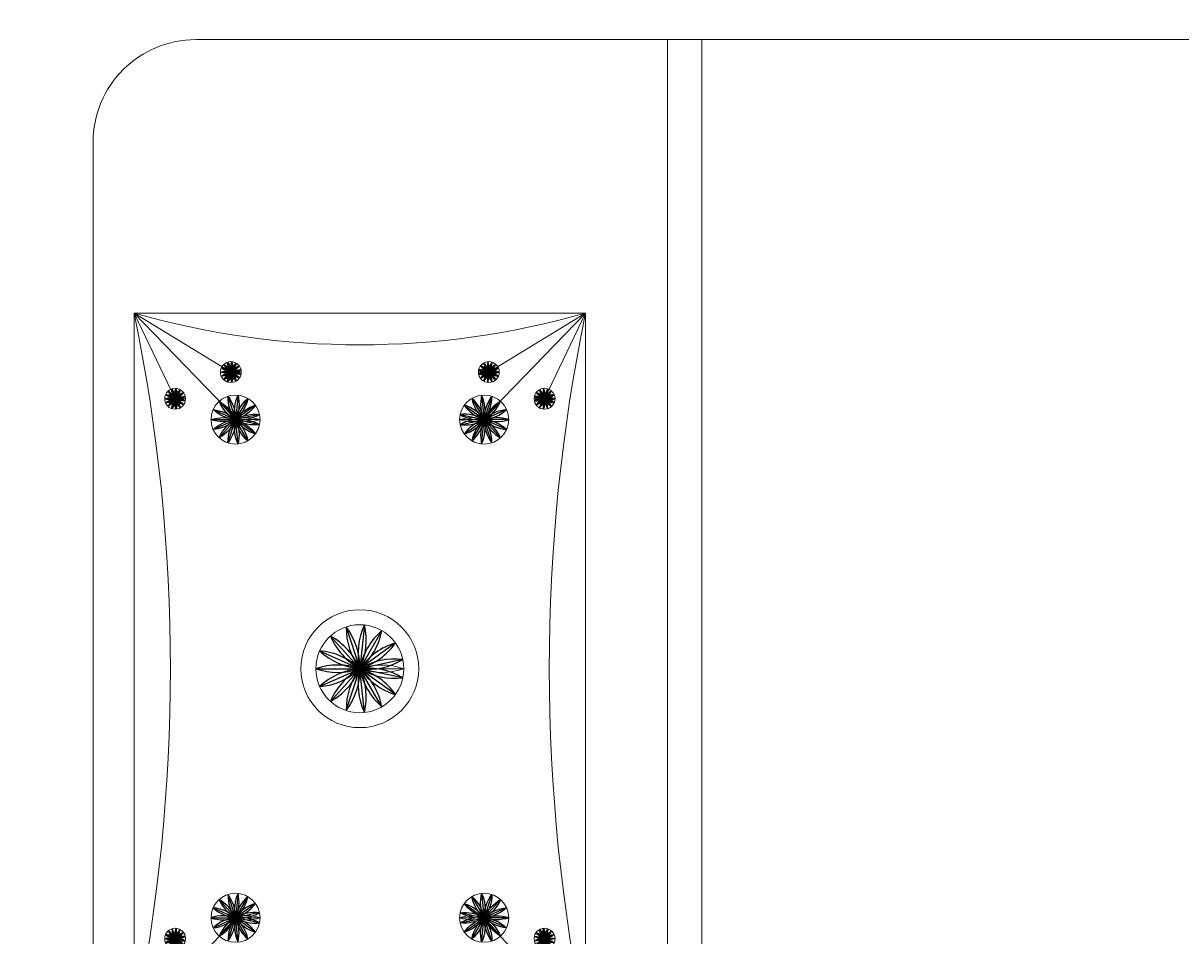
# Model space of a CAD drawing. Units: inches. Extents: x -61 to 1599, y -1316 to 257.
# Tile 149 of 204: x 406 to 440, y 101 to 127. Entities that reach past the tile are written whole.
import ezdxf

# ---------------------------------------------------------------- set-up
doc = ezdxf.new("R2010")
doc.units = ezdxf.units.IN
doc.header["$MEASUREMENT"] = 0
doc.layers.add('A-ANNO-DIMS', color=2, linetype='Continuous', lineweight=18)
doc.layers.add('FURNITURE', color=83, linetype='Continuous', lineweight=18)
doc.layers.add('LT', color=8, linetype='Continuous')
doc.styles.get("Standard").update_dxf_attribs({"font": 'arial.ttf'})
doc.dimstyles.get("Standard").update_dxf_attribs({"dimtxt": 0.18, "dimasz": 0.18, "dimexe": 0.18, "dimexo": 0.0625, "dimgap": 0.09, "dimtad": 0, "dimtih": 1, "dimtoh": 1, "dimdec": 0, "dimzin": 0, "dimdsep": 46, "dimlunit": 3, "dimtxsty": 'Standard', "dimcen": 0.09, "dimadec": 0, "dimazin": 0, "dimtfac": 1, "dimtdec": 0, "dimtofl": 0, "dimtmove": 0, "dimatfit": 3, "dimfxl": 1, "dimtolj": 1, "dimtzin": 0, "dimarcsym": 0})

# ---------------------------------------------------------------- blocks, each defined once
blk = doc.blocks.new('*U71')
at = {"layer": 'LT'}
blk.add_line((0, 0.152), (0, -0.152), dxfattribs=at)
for centre, start, end in [((0.443, 0), 160.9983, 199.0017), ((-0.443, 0), 340.9983, 19.0017)]:
    blk.add_arc(centre, 0.468, start, end, dxfattribs=at)
blk = doc.blocks.new('*U58')
at = {"layer": 'LT', "transparency": 16777216}
for p, rotation in [((-57.958, -16.311), 72), ((-57.926, -16.256), 48.00000000000001), ((-57.875, -16.219), 24), ((-57.751, -16.219), 336), ((-57.699, -16.256), 312), ((-57.668, -16.311), 288), ((-57.964, -16.374), 96), ((-57.945, -16.435), 120), ((-57.902, -16.482), 144), ((-57.844, -16.508), 168.0000000000001), ((-57.781, -16.508), 192), ((-57.723, -16.482), 216), ((-57.68, -16.435), 240), ((-57.661, -16.374), 264)]:
    blk.add_blockref('*U71', p, dxfattribs=dict(at, rotation=rotation))
blk.add_blockref('*U71', (-57.813, -16.206), dxfattribs=at)
blk = doc.blocks.new('*U61')
at = {"layer": 'LT'}
blk.add_line((0, 0.152), (0, -0.152), dxfattribs=at)
for centre, start, end in [((0.443, 0), 160.9983, 199.0017), ((-0.443, 0), 340.9983, 19.0017)]:
    blk.add_arc(centre, 0.468, start, end, dxfattribs=at)
blk = doc.blocks.new('*U62')
at = {"layer": 'LT', "transparency": 16777216}
for p, rotation in [((-57.958, -16.311), 72), ((-57.926, -16.256), 48.00000000000001), ((-57.875, -16.219), 24), ((-57.751, -16.219), 336), ((-57.699, -16.256), 312), ((-57.668, -16.311), 288), ((-57.964, -16.374), 96), ((-57.945, -16.435), 120), ((-57.902, -16.482), 144), ((-57.844, -16.508), 168.0000000000001), ((-57.781, -16.508), 192), ((-57.723, -16.482), 216), ((-57.68, -16.435), 240), ((-57.661, -16.374), 264)]:
    blk.add_blockref('*U61', p, dxfattribs=dict(at, rotation=rotation))
blk.add_blockref('*U61', (-57.813, -16.206), dxfattribs=at)
blk = doc.blocks.new('*U80')
at = {"layer": 'LT'}
blk.add_line((0, 0.359), (0, -0.359), dxfattribs=at)
for centre, start, end in [((1.041, 0), 160.9983, 199.0017), ((-1.041, 0), 340.9983, 19.0017)]:
    blk.add_arc(centre, 1.101, start, end, dxfattribs=at)
blk = doc.blocks.new('*U96')
at = {"layer": 'LT', "transparency": 16777216}
for p, rotation in [((-136.107, -38.143), 23.99999999999999), ((-135.815, -38.143), 336.0000000000001), ((-136.302, -38.36), 72), ((-136.227, -38.231), 48.00000000000001), ((-135.694, -38.231), 312), ((-135.62, -38.36), 288.0000000000001), ((-136.318, -38.508), 96), ((-136.271, -38.65), 120), ((-136.172, -38.761), 144), ((-136.035, -38.822), 168.0000000000001), ((-135.886, -38.822), 191.9999999999999), ((-135.75, -38.761), 216), ((-135.65, -38.65), 240), ((-135.604, -38.508), 264)]:
    blk.add_blockref('*U80', p, dxfattribs=dict(at, rotation=rotation))
blk.add_blockref('*U80', (-135.961, -38.112), dxfattribs=at)
blk = doc.blocks.new('*U69')
at = {"layer": 'LT'}
blk.add_line((0, 0.359), (0, -0.359), dxfattribs=at)
for centre, start, end in [((1.041, 0), 160.9983, 199.0017), ((-1.041, 0), 340.9983, 19.0017)]:
    blk.add_arc(centre, 1.101, start, end, dxfattribs=at)
blk = doc.blocks.new('*U70')
at = {"layer": 'LT', "transparency": 16777216}
for p, rotation in [((-136.107, -38.143), 23.99999999999999), ((-135.815, -38.143), 336.0000000000001), ((-136.302, -38.36), 72), ((-136.227, -38.231), 48.00000000000001), ((-135.694, -38.231), 312), ((-135.62, -38.36), 288.0000000000001), ((-136.318, -38.508), 96), ((-136.271, -38.65), 120), ((-136.172, -38.761), 144), ((-136.035, -38.822), 168.0000000000001), ((-135.886, -38.822), 191.9999999999999), ((-135.75, -38.761), 216), ((-135.65, -38.65), 240), ((-135.604, -38.508), 264)]:
    blk.add_blockref('*U69', p, dxfattribs=dict(at, rotation=rotation))
blk.add_blockref('*U69', (-135.961, -38.112), dxfattribs=at)
blk = doc.blocks.new('*U67')
at = {"layer": 'LT'}
blk.add_line((0, 0.152), (0, -0.152), dxfattribs=at)
for centre, start, end in [((0.443, 0), 160.9983, 199.0017), ((-0.443, 0), 340.9983, 19.0017)]:
    blk.add_arc(centre, 0.468, start, end, dxfattribs=at)
blk = doc.blocks.new('*U68')
at = {"layer": 'LT', "transparency": 16777216}
for p, rotation in [((-57.958, -16.311), 72), ((-57.926, -16.256), 48.00000000000001), ((-57.875, -16.219), 24), ((-57.751, -16.219), 336), ((-57.699, -16.256), 312), ((-57.668, -16.311), 288), ((-57.964, -16.374), 96), ((-57.945, -16.435), 120), ((-57.902, -16.482), 144), ((-57.844, -16.508), 168.0000000000001), ((-57.781, -16.508), 192), ((-57.723, -16.482), 216), ((-57.68, -16.435), 240), ((-57.661, -16.374), 264)]:
    blk.add_blockref('*U67', p, dxfattribs=dict(at, rotation=rotation))
blk.add_blockref('*U67', (-57.813, -16.206), dxfattribs=at)
blk = doc.blocks.new('*U63')
at = {"layer": 'LT'}
blk.add_line((0, 0.643), (0, -0.643), dxfattribs=at)
for centre, start, end in [((1.867, 0), 160.9983, 199.0017), ((-1.867, 0), 340.9983, 19.0017)]:
    blk.add_arc(centre, 1.975, start, end, dxfattribs=at)
blk = doc.blocks.new('*U64')
at = {"layer": 'LT', "transparency": 16777216}
blk.add_blockref('*U63', (-243.723, -68.32), dxfattribs=at)
for p, rotation in [((-244.201, -68.532), 48.00000000000001), ((-243.984, -68.375), 23.99999999999999), ((-243.461, -68.375), 336.0000000000001), ((-243.245, -68.532), 312), ((-244.334, -68.764), 72), ((-243.111, -68.764), 288), ((-244.362, -69.03), 96), ((-244.28, -69.284), 120), ((-244.101, -69.483), 144), ((-243.856, -69.591), 168), ((-243.589, -69.591), 192), ((-243.345, -69.483), 216), ((-243.166, -69.284), 240), ((-243.083, -69.03), 264)]:
    blk.add_blockref('*U63', p, dxfattribs=dict(at, rotation=rotation))
blk = doc.blocks.new('*U65')
at = {"layer": 'LT'}
blk.add_line((0, 0.359), (0, -0.359), dxfattribs=at)
for centre, start, end in [((1.041, 0), 160.9983, 199.0017), ((-1.041, 0), 340.9983, 19.0017)]:
    blk.add_arc(centre, 1.101, start, end, dxfattribs=at)
blk = doc.blocks.new('*U66')
at = {"layer": 'LT', "transparency": 16777216}
for p, rotation in [((-136.107, -38.143), 23.99999999999999), ((-135.815, -38.143), 336.0000000000001), ((-136.302, -38.36), 72), ((-136.227, -38.231), 48.00000000000001), ((-135.694, -38.231), 312), ((-135.62, -38.36), 288.0000000000001), ((-136.318, -38.508), 96), ((-136.271, -38.65), 120), ((-136.172, -38.761), 144), ((-136.035, -38.822), 168.0000000000001), ((-135.886, -38.822), 191.9999999999999), ((-135.75, -38.761), 216), ((-135.65, -38.65), 240), ((-135.604, -38.508), 264)]:
    blk.add_blockref('*U65', p, dxfattribs=dict(at, rotation=rotation))
blk.add_blockref('*U65', (-135.961, -38.112), dxfattribs=at)
blk = doc.blocks.new('*U85')
at = {"layer": 'LT'}
blk.add_line((0, 0.359), (0, -0.359), dxfattribs=at)
for centre, start, end in [((1.041, 0), 160.9983, 199.0017), ((-1.041, 0), 340.9983, 19.0017)]:
    blk.add_arc(centre, 1.101, start, end, dxfattribs=at)
blk = doc.blocks.new('*U86')
at = {"layer": 'LT', "transparency": 16777216}
for p, rotation in [((-136.107, -38.143), 23.99999999999999), ((-135.815, -38.143), 336.0000000000001), ((-136.302, -38.36), 72), ((-136.227, -38.231), 48.00000000000001), ((-135.694, -38.231), 312), ((-135.62, -38.36), 288.0000000000001), ((-136.318, -38.508), 96), ((-136.271, -38.65), 120), ((-136.172, -38.761), 144), ((-136.035, -38.822), 168.0000000000001), ((-135.886, -38.822), 191.9999999999999), ((-135.75, -38.761), 216), ((-135.65, -38.65), 240), ((-135.604, -38.508), 264)]:
    blk.add_blockref('*U85', p, dxfattribs=dict(at, rotation=rotation))
blk.add_blockref('*U85', (-135.961, -38.112), dxfattribs=at)
blk = doc.blocks.new('*U97')
at = {"layer": 'LT'}
blk.add_line((0, 0.152), (0, -0.152), dxfattribs=at)
for centre, start, end in [((0.443, 0), 160.9983, 199.0017), ((-0.443, 0), 340.9983, 19.0017)]:
    blk.add_arc(centre, 0.468, start, end, dxfattribs=at)
blk = doc.blocks.new('*U98')
at = {"layer": 'LT', "transparency": 16777216}
for p, rotation in [((-57.958, -16.311), 72), ((-57.926, -16.256), 48.00000000000001), ((-57.875, -16.219), 24), ((-57.751, -16.219), 336), ((-57.699, -16.256), 312), ((-57.668, -16.311), 288), ((-57.964, -16.374), 96), ((-57.945, -16.435), 120), ((-57.902, -16.482), 144), ((-57.844, -16.508), 168.0000000000001), ((-57.781, -16.508), 192), ((-57.723, -16.482), 216), ((-57.68, -16.435), 240), ((-57.661, -16.374), 264)]:
    blk.add_blockref('*U97', p, dxfattribs=dict(at, rotation=rotation))
blk.add_blockref('*U97', (-57.813, -16.206), dxfattribs=at)
blk = doc.blocks.new('*U87')
at = {"layer": 'LT'}
blk.add_line((0, 0.152), (0, -0.152), dxfattribs=at)
for centre, start, end in [((0.443, 0), 160.9983, 199.0017), ((-0.443, 0), 340.9983, 19.0017)]:
    blk.add_arc(centre, 0.468, start, end, dxfattribs=at)
blk = doc.blocks.new('*U88')
at = {"layer": 'LT', "transparency": 16777216}
for p, rotation in [((-57.958, -16.311), 72), ((-57.926, -16.256), 48.00000000000001), ((-57.875, -16.219), 24), ((-57.751, -16.219), 336), ((-57.699, -16.256), 312), ((-57.668, -16.311), 288), ((-57.964, -16.374), 96), ((-57.945, -16.435), 120), ((-57.902, -16.482), 144), ((-57.844, -16.508), 168.0000000000001), ((-57.781, -16.508), 192), ((-57.723, -16.482), 216), ((-57.68, -16.435), 240), ((-57.661, -16.374), 264)]:
    blk.add_blockref('*U87', p, dxfattribs=dict(at, rotation=rotation))
blk.add_blockref('*U87', (-57.813, -16.206), dxfattribs=at)
blk = doc.blocks.new('*U91')
at = {"layer": 'LT'}
blk.add_line((0, 0.152), (0, -0.152), dxfattribs=at)
for centre, start, end in [((0.443, 0), 160.9983, 199.0017), ((-0.443, 0), 340.9983, 19.0017)]:
    blk.add_arc(centre, 0.468, start, end, dxfattribs=at)
blk = doc.blocks.new('*U92')
at = {"layer": 'LT', "transparency": 16777216}
for p, rotation in [((-57.958, -16.311), 72), ((-57.926, -16.256), 48.00000000000001), ((-57.875, -16.219), 24), ((-57.751, -16.219), 336), ((-57.699, -16.256), 312), ((-57.668, -16.311), 288), ((-57.964, -16.374), 96), ((-57.945, -16.435), 120), ((-57.902, -16.482), 144), ((-57.844, -16.508), 168.0000000000001), ((-57.781, -16.508), 192), ((-57.723, -16.482), 216), ((-57.68, -16.435), 240), ((-57.661, -16.374), 264)]:
    blk.add_blockref('*U91', p, dxfattribs=dict(at, rotation=rotation))
blk.add_blockref('*U91', (-57.813, -16.206), dxfattribs=at)
blk = doc.blocks.new('BED-DOUBLE-COMPACT')
for p, q in [((16.8, 60.036), (16.8, 0.036)), ((17.8, 60.036), (17.8, 0.036)), ((1.2, 52.036), (14.4, 52.036)), ((1.2, 52.036), (2.398, 49.532)), ((1.2, 52.036), (4.201, 48.934)), ((1.2, 52.036), (4.028, 50.312)), ((14.4, 52.036), (11.4, 48.934)), ((14.4, 52.036), (11.572, 50.312)), ((14.4, 52.036), (13.203, 49.532)), ((14.4, 31.236), (14.4, 52.036)), ((4.028, 50.312), (4.333, 50.312)), ((11.572, 50.312), (11.267, 50.312)), ((2.398, 49.532), (2.703, 49.532)), ((13.203, 49.532), (12.898, 49.532)), ((4.165, 48.922), (4.882, 48.922)), ((11.436, 48.922), (10.719, 48.922)), ((7.8, 41.636), (9.086, 41.636)), ((1.2, 31.236), (4.201, 34.339)), ((4.165, 34.351), (4.882, 34.351)), ((11.436, 34.351), (10.719, 34.351)), ((14.4, 31.236), (11.4, 34.339))]:
    blk.add_line(p, q)
for points in [[(77, 60.036), (3, 60.036, 0.414214), (0, 57.036), (0, 3.036, 0.414214), (3, 0.036), (77, 0.036, 0.414214), (80, 3.036), (80, 57.036, 0.414214)], [(4.333, 50.312, 0.167358), (4.028, 50.312, 0.167358)], [(11.572, 50.312, 0.167358), (11.267, 50.312, 0.167358)], [(2.703, 49.532, 0.167358), (2.398, 49.532, 0.167358)], [(13.203, 49.532, 0.167358), (12.898, 49.532, 0.167358)], [(4.882, 48.922, 0.167358), (4.165, 48.922, 0.167358)], [(11.436, 48.922, 0.167358), (10.719, 48.922, 0.167358)], [(7.8, 41.636, 0.167358), (9.086, 41.636, 0.167358)], [(4.165, 34.351, 0.167358), (4.882, 34.351, 0.167358)], [(10.719, 34.351, 0.167358), (11.436, 34.351, 0.167358)]]:
    blk.add_lwpolyline(points, format="xyb", close=True)
blk.add_lwpolyline([(14.4, 31.236), (1.2, 31.236), (1.2, 52.036), (14.4, 52.036), (14.4, 31.236), (1.2, 31.236), (1.2, 52.036)])
for centre, radius in [((4.028, 50.312), 0.305), ((11.572, 50.312), 0.305), ((2.398, 49.532), 0.305), ((13.203, 49.532), 0.305), ((4.165, 48.922), 0.717), ((11.436, 48.922), 0.717), ((7.8, 41.636), 1.724), ((7.8, 41.636), 1.286), ((4.165, 34.351), 0.717), ((11.436, 34.351), 0.717), ((2.398, 33.74), 0.305), ((13.203, 33.74), 0.305)]:
    blk.add_circle(centre, radius)
for centre, radius, start, end in [((-49.227, 41.636), 51.488, 348.3468, 11.6532), ((7.8, 75.06), 23.951, 254.0046, 285.9954), ((64.827, 41.636), 51.488, 168.3468, 191.6532)]:
    blk.add_arc(centre, radius, start, end)
at = {"xscale": -1}
for name, p, rotation in [('*U68', (-12.33, -7.501), 90), ('*U62', (-13.96, -8.28), 90), ('*U70', (-34.306, -87.039), 90), ('*U66', (49.907, 170.312), 270), ('*U88', (29.561, 91.553), 270)]:
    blk.add_blockref(name, p, dxfattribs=dict(at, rotation=rotation))
for name, p, rotation in [('*U98', (27.931, -7.501), 270), ('*U92', (29.561, -8.28), 270), ('*U86', (49.907, -87.039), 270), ('*U64', (-61.162, 285.359), 89.99999999999999), ('*U96', (-34.306, 170.312), 89.99999999999999), ('*U58', (-13.96, 91.553), 89.99999999999999)]:
    blk.add_blockref(name, p, dxfattribs=dict(rotation=rotation))
blk = doc.blocks.new('*D703')
at = {"layer": 'A-ANNO-DIMS', "color": 0, "lineweight": -2, "transparency": 16777216}
for p, q in [((372.32, -616.882), (372.32, 257.457)), ((455.833, -616.882), (455.833, 257.457)), ((372.5, 257.277), (413.7, 257.277)), ((455.653, 257.277), (414.453, 257.277))]:
    blk.add_line(p, q, dxfattribs=at)
at = {"layer": 'A-ANNO-DIMS', "color": 0, "transparency": 16777216}
for points in [[(372.5, 257.307), (372.5, 257.247), (372.32, 257.277)], [(455.653, 257.307), (455.653, 257.247), (455.833, 257.277)]]:
    blk.add_solid(points, dxfattribs=at)
at = {"layer": 'DEFPOINTS', "color": 0, "transparency": 16777216}
for p in [(455.833, 257.277), (372.32, -616.945), (455.833, -616.945)]:
    blk.add_point(p, dxfattribs=at)
at = {"layer": 'A-ANNO-DIMS', "color": 0, "transparency": 16777216, "insert": (414.076, 257.277), "char_height": 0.18, "attachment_point": 5}
blk.add_mtext('\\A1;83.51', dxfattribs=at)

msp = doc.modelspace()

# ---------------------------------------------------------------- block references
at = {"layer": 'FURNITURE'}
msp.add_blockref('BED-DOUBLE-COMPACT', (407.794, 66.733), dxfattribs=at)

# ---------------------------------------------------------------- dimensions: what is measured, and where the dimension line sits
at = {"layer": 'A-ANNO-DIMS'}
dim = msp.add_linear_dim(base=(455.8327, 257.2771), p1=(372.3201, -616.9446), p2=(455.8327, -616.9446), dimstyle='Standard', override={"dimdec": 2, "dimlfac": 1, "dimrnd": 0, "dimzin": 0, "dimdsep": 46, "dimlunit": 2}, dxfattribs=at)
dim.commit()
dim.dimension.update_dxf_attribs({"geometry": '*D703', "text_midpoint": (414.0764, 257.2771)})

doc.saveas('drawing.dxf')
